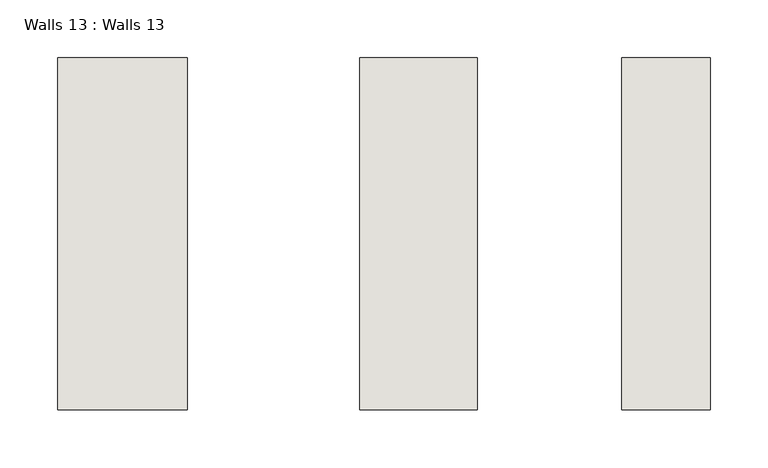
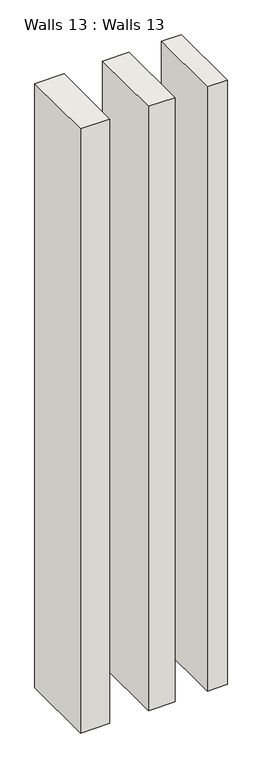
"""IFC4 building model written with IfcOpenShell, lengths in millimetres: wall geometry, Walls 13 : Walls 13."""

from ifc_helpers import new_model, si_unit, frame, origin, place, context, project, spatial, polyline, outline, extrude, source, transform, mapped, element, save


def walls_13_walls_13_063eef50(model_context):
    return source(origin(), model_context, "Body", "SweptSolid", [
        extrude(outline(polyline([(-6452.6407032, 2946.5956099), (-6529.1407032, 2946.5956099), (-6529.1407032, 3251.3956099), (-6452.6407032, 3251.3956099), (-6452.6407032, 2946.5956099)])), frame((0.0, 0.0, 3048.0), z_axis=(0.0, 0.0, 1.0), x_axis=(1.0, 0.0, 0.0)), (0.0, 0.0, 1.0), 2457.1455997),
        extrude(outline(polyline([(-6654.5659632, 2946.5956099), (-6756.1407032, 2946.5956099), (-6756.1407032, 3251.3956099), (-6654.5659632, 3251.3956099), (-6654.5659632, 2946.5956099)])), frame((0.0, 0.0, 3048.0), z_axis=(0.0, 0.0, 1.0), x_axis=(1.0, 0.0, 0.0)), (0.0, 0.0, 1.0), 2457.1455997),
        extrude(outline(polyline([(-6905.7284293, 2946.5956099), (-7017.6924202, 2946.5956099), (-7017.6924202, 3251.3956099), (-6905.7284293, 3251.3956099), (-6905.7284293, 2946.5956099)])), frame((0.0, 0.0, 3048.0), z_axis=(0.0, 0.0, 1.0), x_axis=(1.0, 0.0, 0.0)), (0.0, 0.0, 1.0), 2457.1455997),
    ])


if __name__ == "__main__":
    model = new_model("IFC4")
    model_context = context("Model", 3, world=origin())
    ifc_project = project(units=[si_unit("LENGTHUNIT", "METRE", prefix="MILLI")], contexts=[model_context])
    site = spatial("IfcSite", under=ifc_project)
    building = spatial("IfcBuilding", under=site)
    placement = place(None, origin())
    walls_13_walls_13_shape = walls_13_walls_13_063eef50(model_context)
    element("IfcWall", 1, ObjectType="Walls 13 : Walls 13", at=placement, inside=building, context=model_context, shape_type="MappedRepresentation", body=[
        mapped(walls_13_walls_13_shape, transform((0.0, 0.0, 0.0), x_axis=(1.0, 0.0, 0.0), y_axis=(0.0, 1.0, 0.0), z_axis=(0.0, 0.0, 1.0))),
    ])
    save(model, "model.ifc")

# Revit data of these elements
# Element 1 (IfcWall, "Walls 13 : Walls 13")
#   Materials on its faces: "Default Wall"
# Materials
#   "Default Wall": colour RGB 80 80 80, transparency 0
